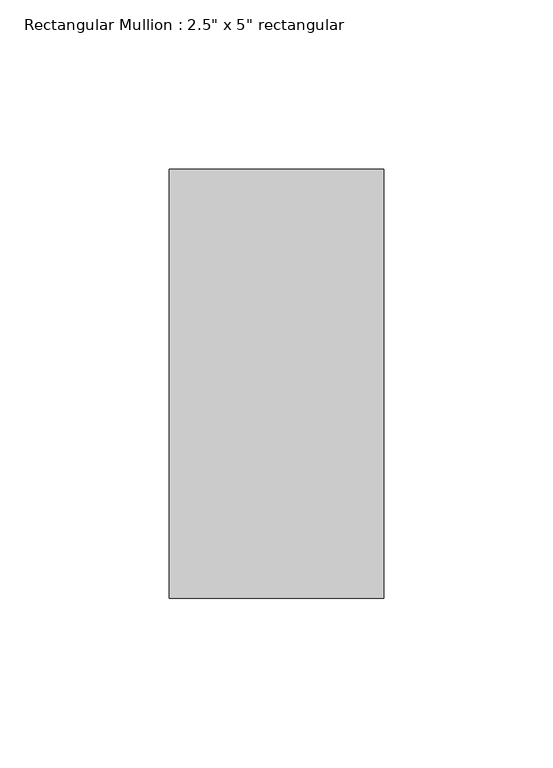
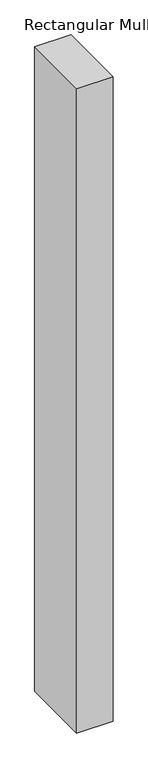
"""IFC4 building model written with IfcOpenShell, lengths in millimetres: member geometry."""

from ifc_helpers import new_model, si_unit, frame, origin, place, context, project, spatial, polyline, outline, extrude, source, transform, mapped, element, save


def member_b3f2e294(model_context):
    return source(origin(), model_context, "Body", "SweptSolid", [
        extrude(outline(polyline([(31.75, 63.5), (31.75, -63.5), (-31.75, -63.5), (-31.75, 63.5), (31.75, 63.5)])), frame((0.0, 0.0, -1187.45), z_axis=(0.0, 0.0, 1.0), x_axis=(1.0, 0.0, 0.0)), (0.0, 0.0, 1.0), 1187.45),
    ])


if __name__ == "__main__":
    model = new_model("IFC4")
    model_context = context("Model", 3, world=origin())
    ifc_project = project(units=[si_unit("LENGTHUNIT", "METRE", prefix="MILLI")], contexts=[model_context])
    site = spatial("IfcSite", under=ifc_project)
    building = spatial("IfcBuilding", under=site)
    placement = place(None, origin())
    member_shape = member_b3f2e294(model_context)
    element("IfcMember", 1, ObjectType="Rectangular Mullion : 2.5\" x 5\" rectangular", at=placement, inside=building, context=model_context, shape_type="MappedRepresentation", body=[
        mapped(member_shape, transform((0.0, 0.0, 0.0), x_axis=(1.0, 0.0, 0.0), y_axis=(0.0, 1.0, 0.0), z_axis=(0.0, 0.0, 1.0))),
    ])
    save(model, "model.ifc")

# Revit data of these elements
# Type "Rectangular Mullion : 2.5\" x 5\" rectangular"
#   built-in parameter 1007304 = 0.416667 (stored number, unit not read)
#   built-in parameter 1007301 = 0.104167 (stored number, unit not read)
#   built-in parameter 1007300 = 0.104167 (stored number, unit not read)
# Element 1 (IfcMember, "Rectangular Mullion : 2.5\" x 5\" rectangular")
#   Materials on its faces: "Aluminum"
# Materials
#   "Aluminum": class "Metal", colour RGB 247 247 247, transparency 0, Description = "Aluminum 6061", Cost = 0
